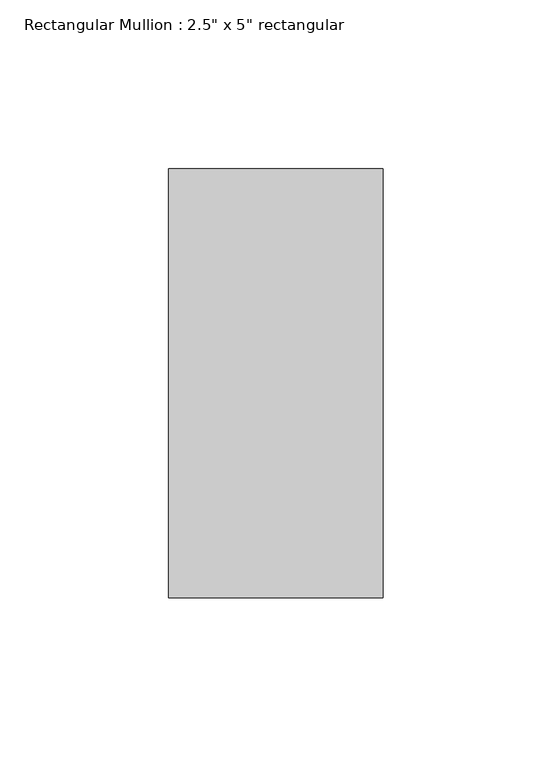
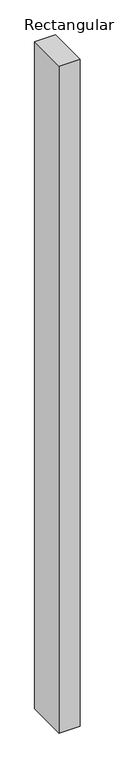
"""IFC4 building model written with IfcOpenShell, lengths in millimetres: member geometry."""

from ifc_helpers import new_model, si_unit, frame, origin, place, context, project, spatial, polyline, outline, extrude, source, transform, mapped, element, save


def member_3e830f4e(model_context):
    return source(origin(), model_context, "Body", "SweptSolid", [
        extrude(outline(polyline([(0.0, 63.5), (0.0, -63.5), (-63.5, -63.5), (-63.5, 63.5), (0.0, 63.5)])), frame((0.0, 0.0, -2129.1310998), z_axis=(0.0, 0.0, 1.0), x_axis=(1.0, 0.0, 0.0)), (0.0, 0.0, 1.0), 2129.1310998),
    ])


if __name__ == "__main__":
    model = new_model("IFC4")
    model_context = context("Model", 3, world=origin())
    ifc_project = project(units=[si_unit("LENGTHUNIT", "METRE", prefix="MILLI")], contexts=[model_context])
    site = spatial("IfcSite", under=ifc_project)
    building = spatial("IfcBuilding", under=site)
    placement = place(None, origin())
    member_shape = member_3e830f4e(model_context)
    element("IfcMember", 1, ObjectType="Rectangular Mullion : 2.5\" x 5\" rectangular", at=placement, inside=building, context=model_context, shape_type="MappedRepresentation", body=[
        mapped(member_shape, transform((0.0, 0.0, 0.0), x_axis=(1.0, 0.0, 0.0), y_axis=(0.0, 1.0, 0.0), z_axis=(0.0, 0.0, 1.0))),
    ])
    save(model, "model.ifc")

# Revit data of these elements
# Type "Rectangular Mullion : 2.5\" x 5\" rectangular"
#   built-in parameter 1007304 = 0.416667 (stored number, unit not read)
#   built-in parameter 1007301 = 0.104167 (stored number, unit not read)
#   built-in parameter 1007300 = 0.104167 (stored number, unit not read)
# Element 1 (IfcMember, "Rectangular Mullion : 2.5\" x 5\" rectangular")
#   Materials on its faces: "Aluminum"
# Materials
#   "Aluminum": class "Metal", colour RGB 247 247 247, transparency 0, Description = "Aluminum 6061", Cost = 0
